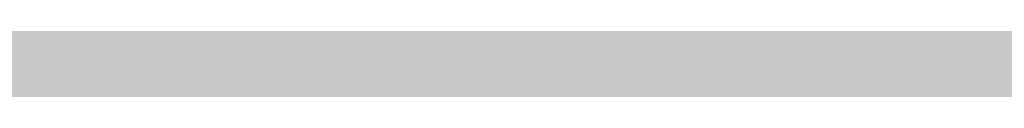
# Model space of a CAD drawing. Units: feet. Extents: x 3168 to 4724, y 827 to 1477.
# Tile 206 of 256: x 3333 to 3364, y 1097 to 1098. Entities that reach past the tile are written whole.
import ezdxf

# ---------------------------------------------------------------- set-up
doc = ezdxf.new("R2010")
doc.units = ezdxf.units.FT
doc.layers.add('A-ELEV-PATT', color=8, linetype='Continuous', lineweight=13)

msp = doc.modelspace()

# ---------------------------------------------------------------- hatches: boundary and pattern name
at = {"layer": 'A-ELEV-PATT'}
h = msp.add_hatch(color=256, dxfattribs=at)
h.dxf.hatch_style = 1
edge = h.paths.add_edge_path()
edge.add_ellipse((3552.906, 979.22), major_axis=(36.745, 0), ratio=0.484848, start_angle=0, end_angle=360)
edge = h.paths.add_edge_path()
edge.add_ellipse((3559.892, 929.252), major_axis=(36.745, 0), ratio=0.484848, start_angle=0, end_angle=360)
edge = h.paths.add_edge_path()
edge.add_line((3299.317, 1198.606), (3479.917, 1198.606))
edge.add_line((3479.917, 1198.606), (3479.917, 1209.869))
edge.add_spline(control_points=[(3479.917, 1209.869), (3464.301, 1209.869), (3448.686, 1209.869), (3410.949, 1209.869), (3388.828, 1209.869), (3355.647, 1209.869), (3344.586, 1209.869), (3327.996, 1209.869), (3322.466, 1209.869), (3314.17, 1209.869), (3311.405, 1209.869), (3307.257, 1209.869), (3305.875, 1209.869), (3303.801, 1209.869), (3303.11, 1209.869), (3302.073, 1209.869), (3301.727, 1209.869), (3301.209, 1209.869), (3301.036, 1209.869), (3300.777, 1209.869), (3300.69, 1209.869), (3300.561, 1209.869), (3300.517, 1209.869), (3300.453, 1209.869), (3300.431, 1209.869), (3300.399, 1209.869), (3300.388, 1209.869), (3300.366, 1209.869), (3300.346, 1209.869), (3300.346, 1209.869), (3300.346, 1209.869), (3300.343, 1209.869), (3300.341, 1209.869), (3300.338, 1209.869), (3300.337, 1209.869), (3300.334, 1209.869), (3300.332, 1209.869), (3300.326, 1209.869), (3300.321, 1209.869), (3300.311, 1209.869), (3300.306, 1209.869), (3300.291, 1209.869), (3300.28, 1209.869), (3300.232, 1209.869), (3300.195, 1209.869), (3299.951, 1209.871), (3299.745, 1209.874), (3299.437, 1209.883), (3299.334, 1209.887), (3299.181, 1209.893), (3299.13, 1209.895), (3298.652, 1209.917), (3298.229, 1209.946), (3297.602, 1210.002), (3297.393, 1210.023), (3297.083, 1210.058), (3296.979, 1210.07), (3296.293, 1210.155), (3295.718, 1210.243), (3294.869, 1210.399), (3294.588, 1210.454), (3294.169, 1210.543), (3294.03, 1210.574), (3291.707, 1211.101), (3289.654, 1211.813), (3285.776, 1213.564), (3283.951, 1214.603), (3280.512, 1216.98), (3278.897, 1218.318), (3276.38, 1220.829), (3275.416, 1221.918), (3274.039, 1223.708), (3273.581, 1224.35), (3273.143, 1225.016)], knot_values=[39.119033, 39.119033, 39.119033, 39.119033, 39.286353, 39.286353, 39.523379, 39.523379, 39.641892, 39.641892, 39.701148, 39.701148, 39.730777, 39.730777, 39.745591, 39.745591, 39.752998, 39.752998, 39.756701, 39.756701, 39.758553, 39.758553, 39.759479, 39.759479, 39.759942, 39.759942, 39.760173, 39.760173, 39.760289, 39.760289, 39.760405, 39.760405, 39.760463, 39.760463, 39.763389, 39.763389, 39.764851, 39.764851, 39.767304, 39.767304, 39.773825, 39.773825, 39.78057, 39.78057, 39.79477, 39.79477, 39.845194, 39.845194, 40.126715, 40.126715, 40.267476, 40.267476, 40.337856, 40.337856, 40.927023, 40.927023, 41.221606, 41.221606, 41.368898, 41.368898, 42.202622, 42.202622, 42.619485, 42.619485, 42.827916, 42.827916, 46.118323, 46.118323, 49.408731, 49.408731, 52.699139, 52.699139, 54.927489, 54.927489, 56.104228, 56.104228, 56.104228, 56.104228], weights=[1, 1, 1, 1, 1, 1, 1, 1, 1, 1, 1, 1, 1, 1, 1, 1, 1, 1, 1, 1, 1, 1, 1, 1, 1, 1, 1, 1, 1, 1, 1, 1, 1, 1, 1, 1, 1, 1, 1, 1, 1, 1, 1, 1, 1, 1, 1, 1, 1, 1, 1, 1, 1, 1, 1, 1, 1, 1, 1, 1, 1, 1, 1, 1, 1, 1, 1, 1, 1, 1, 1, 1, 1, 1], degree=3, periodic=0)
edge.add_line((3273.143, 1225.016), (3273.143, 1099.016))
edge.add_line((3273.143, 1099.016), (3299.317, 1099.016))
edge.add_line((3299.317, 1099.016), (3299.317, 1198.606))
edge = h.paths.add_edge_path()
edge.add_line((3304.758, 1324.158), (3479.917, 1324.158))
edge.add_line((3479.917, 1324.158), (3479.917, 1335.715))
edge.add_line((3479.917, 1335.715), (3269.162, 1335.715))
edge.add_spline(control_points=[(3269.162, 1335.715), (3264.024, 1335.715), (3258.364, 1328.958), (3259.264, 1323.9)], knot_values=[0, 0, 0, 0, 15.412191, 15.412191, 15.412191, 15.412191], degree=3, periodic=0)
edge.add_line((3259.264, 1323.9), (3265.517, 1288.769))
edge.add_line((3265.517, 1288.769), (3275.265, 1261.546))
edge.add_line((3275.265, 1261.546), (3304.758, 1261.546))
edge.add_line((3304.758, 1261.546), (3304.758, 1324.158))
h = msp.add_hatch(color=256, dxfattribs=at)
h.dxf.hatch_style = 1
h.paths.add_polyline_path([(3384.525, 1099.016), (3335.029, 1099.016), (3299.317, 1099.016), (3273.143, 1099.016), (3217.565, 1099.016), (3168.069, 827.116), (3335.029, 827.116)])

doc.saveas('drawing.dxf')
